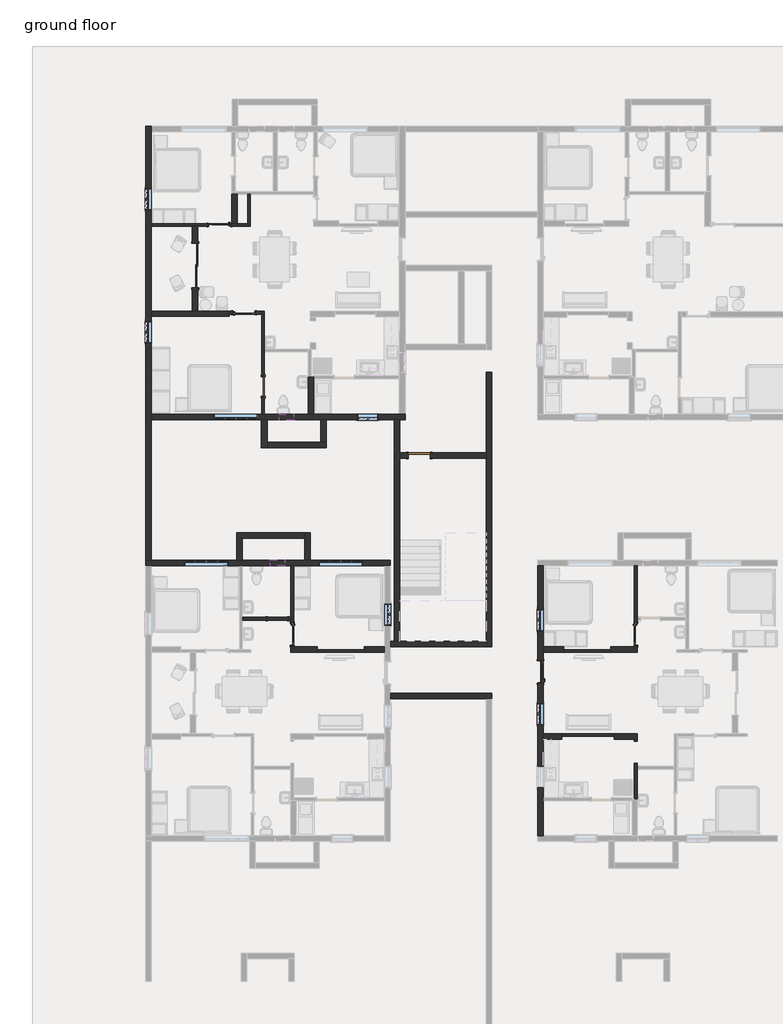
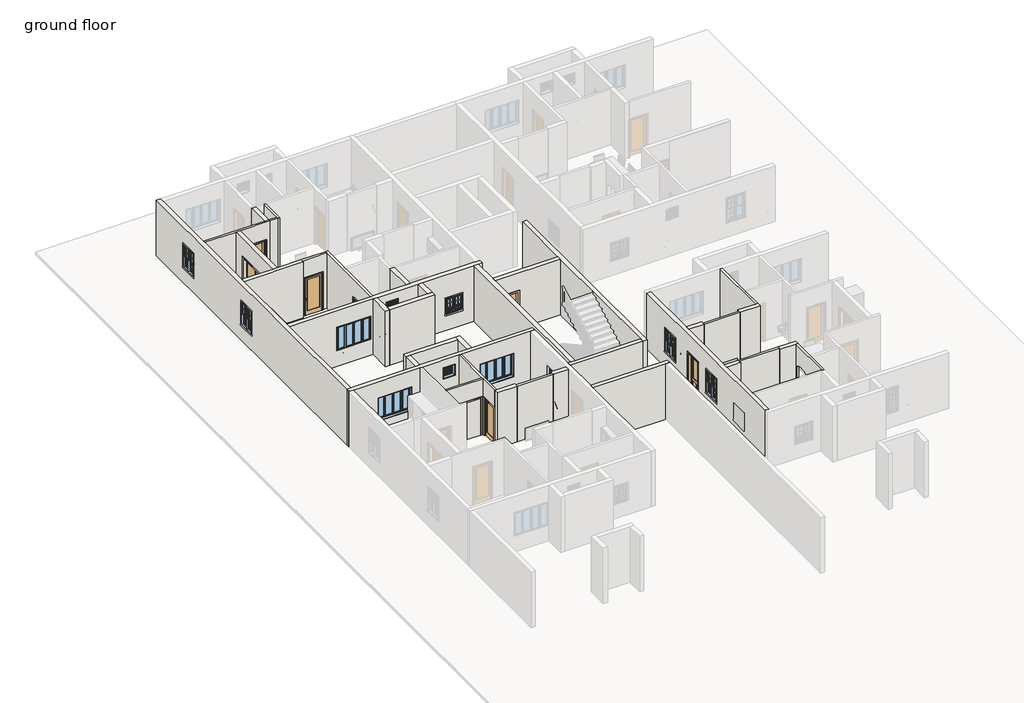
# One storey, part 7 of 16: 38 walls, 11 windows, 9 doors.
"""IFC4 building model written with IfcOpenShell, lengths in millimetres."""

from ifc_helpers import new_model, si_unit, point, frame, origin, place, context, project, spatial, polyline, ellipse_curve, trimmed, outline, extrude, faceted_brep, transform, mapped, element, save
from ifc_brep_helpers import plane_surface, extruded_surface, advanced_brep
from components import door_f079f64e, door_d4d75d1e, door_a3feeac7, door_3c6ab76a, door_38851409, door_a90ba1ad, window_ced37e8f, window_5487fb6d, window_f2d8fef0, window_45970670

model = new_model("IFC4")

# Units and contexts
model_context = context("Model", 3, world=origin())
ifc_project = project(units=[si_unit("LENGTHUNIT", "METRE", prefix="MILLI")], contexts=[model_context])

# Site, building, storey
site = spatial("IfcSite", under=ifc_project)
building = spatial("IfcBuilding", under=site)
storey = spatial("IfcBuildingStorey", under=building, Name="ground floor", Elevation=609.6)

# Doors
placement = place(None, origin())
door_shape = door_f079f64e(model_context)
element("IfcDoor", 1, ObjectType="36\" x 84\"", at=placement, inside=storey, context=model_context, shape_type="MappedRepresentation", body=[
    mapped(door_shape, transform((59474.0062819, 28018.8650652, 609.6), x_axis=(0.0, -1.0, 0.0), y_axis=(1.0, 0.0, 0.0), z_axis=(0.0, 0.0, 1.0))),
])
door_2_shape = door_d4d75d1e(model_context)
element("IfcDoor", 2, ObjectType="Door-Double-Sliding : 72\" x 84\"", at=placement, inside=storey, context=model_context, shape_type="MappedRepresentation", body=[
    mapped(door_2_shape, transform((45068.5142308, 44814.5310851, 609.6), x_axis=(0.0, -1.0, 0.0), y_axis=(1.0, 0.0, 0.0), z_axis=(0.0, 0.0, 1.0))),
])
door_3_shape = door_a3feeac7(model_context)
element("IfcDoor", 3, ObjectType="Door-Interior-Single-1_Panel-Wood : 36\" x 84\"", at=placement, inside=storey, context=model_context, shape_type="MappedRepresentation", body=[
    mapped(door_3_shape, transform((46206.3837344, 46494.1060851, 609.6), x_axis=(-1.0, 0.0, 0.0), y_axis=(0.0, -1.0, 0.0), z_axis=(0.0, 0.0, 1.0))),
])
element("IfcDoor", 4, ObjectType="Door-Interior-Single-1_Panel-Wood : 36\" x 84\"", at=placement, inside=storey, context=model_context, shape_type="MappedRepresentation", body=[
    mapped(door_3_shape, transform((47204.5368314, 42863.06804, 609.6), x_axis=(1.0, 0.0, 0.0), y_axis=(0.0, 1.0, 0.0), z_axis=(0.0, 0.0, 1.0))),
])
element("IfcDoor", 5, ObjectType="Door-Interior-Single-1_Panel-Wood : 36\" x 84\"", at=placement, inside=storey, context=model_context, shape_type="MappedRepresentation", body=[
    mapped(door_3_shape, transform((63411.0062819, 29571.4400652, 609.6), x_axis=(0.0, -1.0, 0.0), y_axis=(1.0, 0.0, 0.0), z_axis=(0.0, 0.0, 1.0))),
])
door_4_shape = door_3c6ab76a(model_context)
element("IfcDoor", 6, ObjectType="Door-Interior-Single-1_Panel-Wood : 36\" x 84\"", at=placement, inside=storey, context=model_context, shape_type="MappedRepresentation", body=[
    mapped(door_4_shape, transform((49209.051243, 29571.4400652, 609.6), x_axis=(0.0, -1.0, 0.0), y_axis=(1.0, 0.0, 0.0), z_axis=(0.0, 0.0, 1.0))),
])
door_5_shape = door_38851409(model_context)
element("IfcDoor", 7, ObjectType="Single-Flush : 32\" x 84\"", at=placement, inside=storey, context=model_context, shape_type="MappedRepresentation", body=[
    mapped(door_5_shape, transform((47998.2868314, 39817.8809867, 609.6), x_axis=(0.0, 1.0, 0.0), y_axis=(-1.0, 0.0, 0.0), z_axis=(0.0, 0.0, 1.0))),
])
element("IfcDoor", 8, ObjectType="Single-Flush : 32\" x 84\"", at=placement, inside=storey, context=model_context, shape_type="MappedRepresentation", body=[
    mapped(door_5_shape, transform((48596.276243, 30209.6150652, 609.6), x_axis=(-1.0, 0.0, 0.0), y_axis=(0.0, -1.0, 0.0), z_axis=(0.0, 0.0, 1.0))),
])
door_6_shape = door_a90ba1ad(model_context)
element("IfcDoor", 9, ObjectType="Single-Flush : 36\" x 84\"", at=placement, inside=storey, context=model_context, shape_type="MappedRepresentation", body=[
    mapped(door_6_shape, transform((54460.4072437, 36957.8375431, 609.6), x_axis=(-1.0, 0.0, 0.0), y_axis=(0.0, -1.0, 0.0), z_axis=(0.0, 0.0, 1.0))),
])

# Walls
element("IfcWall", 10, ObjectType="Generic - 4.5\"", at=placement, inside=storey, context=model_context, shape_type="Brep", body=[
    faceted_brep([(47941.1368314, 42923.39304, 609.6), (47941.1368314, 42809.09304, 609.6), (47941.1368314, 40224.2809867, 609.6), (47941.1368314, 40224.2809867, 2743.2), (47941.1368314, 39411.4809867, 2743.2), (47941.1368314, 39411.4809867, 609.6), (47941.1368314, 38662.1809867, 609.6), (47941.1368314, 38662.1809867, 3810.0), (47941.1368314, 42809.09304, 3810.0), (47941.1368314, 42923.39304, 3810.0), (48055.4368314, 40224.2809867, 2743.2), (48055.4368314, 40224.2809867, 609.6), (48055.4368314, 41243.6395295, 609.6), (48055.4368314, 41357.9395295, 609.6), (48055.4368314, 42923.39304, 609.6), (48055.4368314, 42923.39304, 3810.0), (48055.4368314, 41357.9395295, 3810.0), (48055.4368314, 41243.6395295, 3810.0), (48055.4368314, 38662.1809867, 3810.0), (48055.4368314, 38662.1809867, 609.6), (48055.4368314, 39411.4809867, 609.6), (48055.4368314, 39411.4809867, 2743.2)], [[[0, 1, 2, 3, 4, 5, 6, 7, 8, 9]], [[10, 11, 12, 13, 14, 15, 16, 17, 18, 19, 20, 21]], [[20, 19, 6, 5]], [[14, 13, 12, 11, 2, 1, 0]], [[9, 8, 7, 18, 17, 16, 15]], [[0, 9, 15, 14]], [[7, 6, 19, 18]], [[3, 2, 11, 10]], [[4, 3, 10, 21]], [[5, 4, 21, 20]]]),
])
element("IfcWall", 11, ObjectType="Generic - 4.5\"", at=placement, inside=storey, context=model_context, shape_type="SweptSolid", body=[
    extrude(outline(polyline([(3810.0, 46594.9368314), (609.6, 46594.9368314), (609.6, 46721.9368314), (2768.6, 46721.9368314), (2768.6, 47687.1368314), (609.6, 47687.1368314), (609.6, 47941.1368314), (3810.0, 47941.1368314), (3810.0, 46594.9368314)])), frame((0.0, 42809.09304, 0.0), z_axis=(0.0, 1.0, 0.0), x_axis=(0.0, 0.0, 1.0)), (0.0, 0.0, 1.0), 114.3),
])
element("IfcWall", 12, ObjectType="Generic - 4.5\"", at=placement, inside=storey, context=model_context, shape_type="Brep", body=[
    faceted_brep([(46930.2837344, 46433.7810851, 3810.0), (45309.8142308, 46433.7810851, 3810.0), (45081.2142308, 46433.7810851, 3810.0), (43370.226243, 46433.7810851, 3810.0), (43370.226243, 46433.7810851, 609.6), (45081.2142308, 46433.7810851, 609.6), (45309.8142308, 46433.7810851, 609.6), (45723.7837344, 46433.7810851, 609.6), (45723.7837344, 46433.7810851, 2768.6), (46688.9837344, 46433.7810851, 2768.6), (46688.9837344, 46433.7810851, 609.6), (46930.2837344, 46433.7810851, 609.6), (43370.226243, 46548.0810851, 3810.0), (46701.6837344, 46548.0810851, 3810.0), (46930.2837344, 46548.0810851, 3810.0), (46930.2837344, 46548.0810851, 609.6), (46701.6837344, 46548.0810851, 609.6), (46688.9837344, 46548.0810851, 609.6), (46688.9837344, 46548.0810851, 2768.6), (45723.7837344, 46548.0810851, 2768.6), (45723.7837344, 46548.0810851, 609.6), (43370.226243, 46548.0810851, 609.6)], [[[0, 1, 2, 3, 4, 5, 6, 7, 8, 9, 10, 11]], [[12, 13, 14, 15, 16, 17, 18, 19, 20, 21]], [[4, 21, 20, 7, 6, 5]], [[15, 11, 10, 17, 16]], [[3, 2, 1, 0, 14, 13, 12]], [[4, 3, 12, 21]], [[0, 11, 15, 14]], [[19, 8, 7, 20]], [[8, 19, 18, 9]], [[9, 18, 17, 10]]]),
])
element("IfcWall", 13, ObjectType="Generic - 4.5\"", at=placement, inside=storey, context=model_context, shape_type="Brep", body=[
    faceted_brep([(47362.0837344, 47759.2773256, 609.6), (47362.0837344, 46547.9632967, 609.6), (47362.0837344, 46433.6632967, 609.6), (47362.0837344, 46433.6632967, 3810.0), (47362.0837344, 46547.9632967, 3810.0), (47362.0837344, 47759.2773256, 3810.0), (47476.3837344, 47759.2773256, 609.6), (47476.3837344, 47759.2773256, 3810.0), (47476.3837344, 46433.6632967, 3810.0), (47476.3837344, 46433.6632967, 609.6)], [[[0, 1, 2, 3, 4, 5]], [[6, 7, 8, 9]], [[2, 1, 0, 6, 9]], [[5, 4, 3, 8, 7]], [[0, 5, 7, 6]], [[3, 2, 9, 8]]]),
])
element("IfcWall", 14, ObjectType="Generic - 4.5\"", at=placement, inside=storey, context=model_context, shape_type="SweptSolid", body=[
    extrude(outline(polyline([(46930.2837344, 46547.9632967), (47362.0837344, 46547.9632967), (47362.0837344, 46433.6632967), (46930.2837344, 46433.6632967), (46930.2837344, 46547.9632967)])), frame((0.0, 0.0, 609.6), z_axis=(0.0, 0.0, 1.0), x_axis=(1.0, 0.0, 0.0)), (0.0, 0.0, 1.0), 3200.4),
])
element("IfcWall", 15, ObjectType="Generic - 4.5\"", at=placement, inside=storey, context=model_context, shape_type="SweptSolid", body=[
    extrude(outline(polyline([(62518.8312819, 25351.8650652), (60347.1312819, 25351.8650652), (60347.1312819, 25466.1650652), (62518.8312819, 25466.1650652), (62518.8312819, 25351.8650652)])), frame((0.0, 0.0, 609.6), z_axis=(0.0, 0.0, 1.0), x_axis=(1.0, 0.0, 0.0)), (0.0, 0.0, 1.0), 3200.4),
])
element("IfcWall", 16, ObjectType="Generic - 4.5\"", at=placement, inside=storey, context=model_context, shape_type="AdvancedBrep", body=[
    advanced_brep(
    [(63357.0312819, 24243.7900652, 2540.0), (63357.0312819, 24243.7900652, 609.6), (63357.0312819, 22811.8650652, 609.6), (63357.0312819, 22754.7150652, 609.6), (63357.0312819, 22754.7150652, 3810.0), (63357.0312819, 22811.8650652, 3810.0), (63357.0312819, 25237.5650652, 3810.0), (63357.0312819, 25237.5650652, 609.6), (63357.0312819, 25158.1900652, 609.6), (63357.0312819, 25158.1900652, 2540.0), (63471.3312819, 22754.7150652, 609.6), (63471.3312819, 23992.9650652, 609.6), (63471.3312819, 24107.2650652, 609.6), (63471.3312819, 24243.7900652, 609.6), (63471.3312819, 24243.7900652, 2540.0), (63471.3312819, 25158.1900652, 2540.0), (63471.3312819, 25158.1900652, 609.6), (63471.3312819, 25237.5650652, 609.6), (63471.3312819, 25237.5650652, 3810.0), (63471.3312819, 24107.2650652, 3810.0), (63471.3312819, 23992.9650652, 3810.0), (63471.3312819, 22754.7150652, 3810.0)],
    [
        (0, 1),
        (1, 2),
        (2, 3),
        (3, 4),
        (4, 5),
        (5, 6),
        (6, 7),
        (7, 8),
        (8, 9),
        (9, 0, ellipse_curve(frame((63357.0312819, 24700.9900652, 2540.0), z_axis=(1.0, 0.0, 0.0), x_axis=(0.0, -1.0, 0.0)), 457.2, 203.2)),
        (10, 11),
        (11, 12),
        (12, 13),
        (13, 14),
        (14, 15, ellipse_curve(frame((63471.3312819, 24700.9900652, 2540.0), z_axis=(-1.0, 0.0, 0.0), x_axis=(0.0, -1.0, 0.0)), 457.2, 203.2)),
        (15, 16),
        (16, 17),
        (17, 18),
        (18, 19),
        (19, 20),
        (20, 21),
        (21, 10),
        (7, 17),
        (16, 8),
        (1, 13),
        (10, 3),
        (21, 4),
        (18, 6),
        (14, 0),
        (9, 15),
    ],
    [
        plane_surface(frame((63357.0312819, 25237.5650652, 609.6), z_axis=(-1.0, 0.0, 0.0), x_axis=(0.0, -1.0, 0.0))),
        plane_surface(frame((63471.3312819, 25237.5650652, 609.6), z_axis=(1.0, 0.0, 0.0), x_axis=(0.0, 1.0, 0.0))),
        plane_surface(frame((63357.0312819, 25351.8650652, 609.6), z_axis=(0.0, 0.0, -1.0), x_axis=(1.0, 0.0, 0.0))),
        plane_surface(frame((63357.0312819, 22754.7150652, 609.6), z_axis=(0.0, -1.0, 0.0), x_axis=(1.0, 0.0, 0.0))),
        plane_surface(frame((63357.0312819, 22754.7150652, 3810.0), z_axis=(0.0, 0.0, 1.0), x_axis=(1.0, 0.0, 0.0))),
        plane_surface(frame((62518.8312819, 25237.5650652, 609.6), z_axis=(0.0, 1.0, 0.0), x_axis=(1.0, 0.0, 0.0))),
        extruded_surface(trimmed(ellipse_curve(frame((63242.7312819, 24700.9900652, 2540.0), z_axis=(-1.0, 0.0, 0.0), x_axis=(0.0, -1.0, 0.0)), 457.2, 203.2), [point((63242.7312819, 24243.7900652, 2540.0))], [point((63242.7312819, 25158.1900652, 2540.0))], True, "CARTESIAN"), (114.30000000000291, 0.0, 0.0), 114.30000000000291),
        plane_surface(frame((63471.3312819, 25158.1900652, 2540.0), z_axis=(0.0, -1.0, 0.0), x_axis=(-1.0, 0.0, 0.0))),
        plane_surface(frame((63471.3312819, 24243.7900652, 609.6), z_axis=(0.0, 1.0, 0.0), x_axis=(-1.0, 0.0, 0.0))),
    ],
    [
        (0, [[1, 2, 3, 4, 5, 6, 7, 8, 9, 10]]),
        (1, [[11, 12, 13, 14, 15, 16, 17, 18, 19, 20, 21, 22]]),
        (2, [[-8, 23, -17, 24]]),
        (2, [[-3, -2, 25, -13, -12, -11, 26]]),
        (3, [[-4, -26, -22, 27]]),
        (4, [[-6, -5, -27, -21, -20, -19, 28]]),
        (5, [[-7, -28, -18, -23]]),
        (6, [[-15, 29, -10, 30]]),
        (7, [[-16, -30, -9, -24]]),
        (8, [[-14, -25, -1, -29]]),
    ],
),
])
element("IfcWall", 17, ObjectType="Generic - 4.5\"", at=placement, inside=storey, context=model_context, shape_type="SweptSolid", body=[
    extrude(outline(polyline([(62384.5498476, 28818.9650652), (60423.3312819, 28818.9650652), (60423.3312819, 28933.2650652), (62384.5498476, 28933.2650652), (62384.5498476, 28818.9650652)])), frame((0.0, 0.0, 609.6), z_axis=(0.0, 0.0, 1.0), x_axis=(1.0, 0.0, 0.0)), (0.0, 0.0, 1.0), 3200.4),
])
element("IfcWall", 18, ObjectType="Generic - 4.5\"", at=placement, inside=storey, context=model_context, shape_type="Brep", body=[
    faceted_brep([(63357.0312819, 29047.5650652, 3810.0), (63357.0312819, 32400.3650652, 3810.0), (63357.0312819, 32400.3650652, 609.6), (63357.0312819, 30054.0400652, 609.6), (63357.0312819, 30054.0400652, 2768.6), (63357.0312819, 29088.8400652, 2768.6), (63357.0312819, 29088.8400652, 609.6), (63357.0312819, 29047.5650652, 609.6), (63471.3312819, 32400.3650652, 3810.0), (63471.3312819, 30266.7650652, 3810.0), (63471.3312819, 30152.4650652, 3810.0), (63471.3312819, 29047.5650652, 3810.0), (63471.3312819, 29047.5650652, 609.6), (63471.3312819, 29088.8400652, 609.6), (63471.3312819, 29088.8400652, 2768.6), (63471.3312819, 30054.0400652, 2768.6), (63471.3312819, 30054.0400652, 609.6), (63471.3312819, 30152.4650652, 609.6), (63471.3312819, 30266.7650652, 609.6), (63471.3312819, 32400.3650652, 609.6)], [[[0, 1, 2, 3, 4, 5, 6, 7]], [[8, 9, 10, 11, 12, 13, 14, 15, 16, 17, 18, 19]], [[2, 19, 18, 17, 16, 3]], [[12, 7, 6, 13]], [[1, 0, 11, 10, 9, 8]], [[0, 7, 12, 11]], [[2, 1, 8, 19]], [[5, 14, 13, 6]], [[14, 5, 4, 15]], [[15, 4, 3, 16]]]),
])
element("IfcWall", 19, ObjectType="Generic - 4.5\"", at=placement, inside=storey, context=model_context, shape_type="Brep", body=[
    faceted_brep([(49148.726243, 29047.5650652, 3810.0), (49148.726243, 30152.4650652, 3810.0), (49148.726243, 30266.7650652, 3810.0), (49148.726243, 32412.9272014, 3810.0), (49148.726243, 32412.9272014, 609.6), (49148.726243, 30266.7650652, 609.6), (49148.726243, 30152.4650652, 609.6), (49148.726243, 30054.0400652, 609.6), (49148.726243, 30054.0400652, 2768.6), (49148.726243, 29088.8400652, 2768.6), (49148.726243, 29088.8400652, 609.6), (49148.726243, 29047.5650652, 609.6), (49263.026243, 32412.9272014, 3810.0), (49263.026243, 29047.5650652, 3810.0), (49263.026243, 29047.5650652, 609.6), (49263.026243, 29088.8400652, 609.6), (49263.026243, 29088.8400652, 2768.6), (49263.026243, 30054.0400652, 2768.6), (49263.026243, 30054.0400652, 609.6), (49263.026243, 32412.9272014, 609.6)], [[[0, 1, 2, 3, 4, 5, 6, 7, 8, 9, 10, 11]], [[12, 13, 14, 15, 16, 17, 18, 19]], [[4, 19, 18, 7, 6, 5]], [[14, 11, 10, 15]], [[3, 2, 1, 0, 13, 12]], [[0, 11, 14, 13]], [[4, 3, 12, 19]], [[9, 16, 15, 10]], [[16, 9, 8, 17]], [[17, 8, 7, 18]]]),
])
element("IfcWall", 20, ObjectType="Generic - 4.5\"", at=placement, inside=storey, context=model_context, shape_type="SweptSolid", body=[
    extrude(outline(polyline([(49148.726243, 30152.4650652), (47142.126243, 30152.4650652), (47142.126243, 30266.7650652), (49148.726243, 30266.7650652), (49148.726243, 30152.4650652)])), frame((0.0, 0.0, 609.6), z_axis=(0.0, 0.0, 1.0), x_axis=(1.0, 0.0, 0.0)), (0.0, 0.0, 1.0), 3200.4),
])
element("IfcWall", 21, ObjectType="Generic - 4.5\"", at=placement, inside=storey, context=model_context, shape_type="SweptSolid", body=[
    extrude(outline(polyline([(52192.1804737, 28818.9650652), (50235.5076773, 28818.9650652), (50235.5076773, 28933.2650652), (52192.1804737, 28933.2650652), (52192.1804737, 28818.9650652)])), frame((0.0, 0.0, 609.6), z_axis=(0.0, 0.0, 1.0), x_axis=(1.0, 0.0, 0.0)), (0.0, 0.0, 1.0), 3200.4),
])
element("IfcWall", 22, ObjectType="Generic - 4.5\"", at=placement, inside=storey, context=model_context, shape_type="SweptSolid", body=[
    extrude(outline(polyline([(609.6, 47142.126243), (609.6, 48189.876243), (2743.2, 48189.876243), (2743.2, 49002.676243), (609.6, 49002.676243), (609.6, 49148.726243), (3810.0, 49148.726243), (3810.0, 47142.126243), (609.6, 47142.126243)])), frame((0.0, 30152.4650652, 0.0), z_axis=(0.0, 1.0, 0.0), x_axis=(0.0, 0.0, 1.0)), (0.0, 0.0, 1.0), 114.3),
])
element("IfcWall", 23, ObjectType="Generic - 8\"", at=placement, inside=storey, context=model_context, shape_type="Brep", body=[
    faceted_brep([(43370.226243, 42720.1903135, 609.6), (46594.9368314, 42720.1903135, 609.6), (46594.9368314, 42720.1903135, 3810.0), (43370.226243, 42720.1903135, 3810.0), (43370.226243, 42923.3903135, 609.6), (43370.226243, 42923.3903135, 3810.0), (45081.2142308, 42923.3903135, 3810.0), (45309.8142308, 42923.3903135, 3810.0), (46594.9368314, 42923.3903135, 3810.0), (46594.9368314, 42923.3903135, 609.6), (45309.8142308, 42923.3903135, 609.6), (45081.2142308, 42923.3903135, 609.6), (46594.9368314, 42809.09304, 609.6), (46594.9368314, 42809.09304, 3810.0)], [[[0, 1, 2, 3]], [[4, 5, 6, 7, 8, 9, 10, 11]], [[1, 0, 4, 11, 10, 9, 12]], [[2, 1, 12, 9, 8, 13]], [[3, 2, 13, 8, 7, 6, 5]], [[0, 3, 5, 4]]]),
])
element("IfcWall", 24, ObjectType="Generic - 9\"", at=placement, inside=storey, context=model_context, shape_type="Brep", body=[
    faceted_brep([(43141.626243, 50583.0390836, 609.6), (43141.626243, 32641.5272014, 609.6), (43141.626243, 32641.5272014, 3810.0), (43141.626243, 50583.0390836, 3810.0), (43141.626243, 41602.5903135, 2844.8), (43141.626243, 41602.5903135, 1524.0), (43141.626243, 42516.9903135, 1524.0), (43141.626243, 42516.9903135, 2844.8), (43141.626243, 47100.5310851, 2844.8), (43141.626243, 47100.5310851, 1524.0), (43141.626243, 48014.9310851, 1524.0), (43141.626243, 48014.9310851, 2844.8), (43370.226243, 50583.0390836, 609.6), (43370.226243, 50583.0390836, 3810.0), (43370.226243, 50354.4390836, 3810.0), (43370.226243, 46548.0810851, 3810.0), (43370.226243, 46433.7810851, 3810.0), (43370.226243, 42923.3903135, 3810.0), (43370.226243, 42720.1903135, 3810.0), (43370.226243, 38662.1809867, 3810.0), (43370.226243, 38433.5809867, 3810.0), (43370.226243, 32641.5272014, 3810.0), (43370.226243, 32641.5272014, 609.6), (43370.226243, 38433.5809867, 609.6), (43370.226243, 38662.1809867, 609.6), (43370.226243, 42720.1903135, 609.6), (43370.226243, 42923.3903135, 609.6), (43370.226243, 46433.7810851, 609.6), (43370.226243, 46548.0810851, 609.6), (43370.226243, 50354.4390836, 609.6), (43370.226243, 41602.5903135, 2844.8), (43370.226243, 42516.9903135, 2844.8), (43370.226243, 42516.9903135, 1524.0), (43370.226243, 41602.5903135, 1524.0), (43370.226243, 47100.5310851, 2844.8), (43370.226243, 48014.9310851, 2844.8), (43370.226243, 48014.9310851, 1524.0), (43370.226243, 47100.5310851, 1524.0)], [[[0, 1, 2, 3], [4, 5, 6, 7], [8, 9, 10, 11]], [[12, 13, 14, 15, 16, 17, 18, 19, 20, 21, 22, 23, 24, 25, 26, 27, 28, 29], [30, 31, 32, 33], [34, 35, 36, 37]], [[1, 0, 12, 29, 28, 27, 26, 25, 24, 23, 22]], [[3, 2, 21, 20, 19, 18, 17, 16, 15, 14, 13]], [[0, 3, 13, 12]], [[5, 4, 30, 33]], [[6, 5, 33, 32]], [[7, 6, 32, 31]], [[4, 7, 31, 30]], [[9, 8, 34, 37]], [[10, 9, 37, 36]], [[11, 10, 36, 35]], [[8, 11, 35, 34]], [[2, 1, 22, 21]]]),
])
element("IfcWall", 25, ObjectType="Generic - 9\"", at=placement, inside=storey, context=model_context, shape_type="Brep", body=[
    faceted_brep([(43370.226243, 38433.5809867, 609.6), (47935.8141396, 38433.5809867, 609.6), (48164.4141396, 38433.5809867, 609.6), (50387.9122064, 38433.5809867, 609.6), (50616.5122064, 38433.5809867, 609.6), (53431.7072437, 38433.5809867, 609.6), (53660.3072437, 38433.5809867, 609.6), (53870.1312819, 38433.5809867, 609.6), (53870.1312819, 38433.5809867, 3810.0), (53660.3072437, 38433.5809867, 3810.0), (53431.7072437, 38433.5809867, 3810.0), (50616.5122064, 38433.5809867, 3810.0), (50387.9122064, 38433.5809867, 3810.0), (48164.4141396, 38433.5809867, 3810.0), (47935.8141396, 38433.5809867, 3810.0), (43370.226243, 38433.5809867, 3810.0), (49269.3141396, 38433.5809867, 3352.8), (49269.3141396, 38433.5809867, 2743.2), (48659.7141396, 38433.5809867, 2743.2), (48659.7141396, 38433.5809867, 3352.8), (45966.2868314, 38433.5809867, 1524.0), (45966.2868314, 38433.5809867, 2870.2), (47795.0868314, 38433.5809867, 2870.2), (47795.0868314, 38433.5809867, 1524.0), (51901.6312819, 38433.5809867, 1524.0), (51901.6312819, 38433.5809867, 2438.4), (52765.2312819, 38433.5809867, 2438.4), (52765.2312819, 38433.5809867, 1524.0), (53870.1312819, 38662.1809867, 609.6), (53641.5312819, 38662.1809867, 609.6), (50099.858718, 38662.1809867, 609.6), (49871.258718, 38662.1809867, 609.6), (48055.4368314, 38662.1809867, 609.6), (47941.1368314, 38662.1809867, 609.6), (43370.226243, 38662.1809867, 609.6), (43370.226243, 38662.1809867, 3810.0), (47941.1368314, 38662.1809867, 3810.0), (48055.4368314, 38662.1809867, 3810.0), (49871.258718, 38662.1809867, 3810.0), (50099.858718, 38662.1809867, 3810.0), (53641.5312819, 38662.1809867, 3810.0), (53870.1312819, 38662.1809867, 3810.0), (49269.3141396, 38662.1809867, 2743.2), (49269.3141396, 38662.1809867, 3352.8), (48659.7141396, 38662.1809867, 3352.8), (48659.7141396, 38662.1809867, 2743.2), (45966.2868314, 38662.1809867, 2870.2), (45966.2868314, 38662.1809867, 1524.0), (47795.0868314, 38662.1809867, 1524.0), (47795.0868314, 38662.1809867, 2870.2), (51901.6312819, 38662.1809867, 2438.4), (51901.6312819, 38662.1809867, 1524.0), (52765.2312819, 38662.1809867, 1524.0), (52765.2312819, 38662.1809867, 2438.4)], [[[0, 1, 2, 3, 4, 5, 6, 7, 8, 9, 10, 11, 12, 13, 14, 15], [16, 17, 18, 19], [20, 21, 22, 23], [24, 25, 26, 27]], [[28, 29, 30, 31, 32, 33, 34, 35, 36, 37, 38, 39, 40, 41], [42, 43, 44, 45], [46, 47, 48, 49], [50, 51, 52, 53]], [[7, 6, 5, 4, 3, 2, 1, 0, 34, 33, 32, 31, 30, 29, 28]], [[15, 14, 13, 12, 11, 10, 9, 8, 41, 40, 39, 38, 37, 36, 35]], [[0, 15, 35, 34]], [[8, 7, 28, 41]], [[17, 16, 43, 42]], [[18, 17, 42, 45]], [[19, 18, 45, 44]], [[16, 19, 44, 43]], [[47, 46, 21, 20]], [[48, 47, 20, 23]], [[49, 48, 23, 22]], [[46, 49, 22, 21]], [[50, 25, 24, 51]], [[51, 24, 27, 52]], [[52, 27, 26, 53]], [[25, 50, 53, 26]]]),
])
element("IfcWall", 26, ObjectType="Generic - 9\"", at=placement, inside=storey, context=model_context, shape_type="SweptSolid", body=[
    extrude(outline(polyline([(43900.1310851, 2743.2), (43900.1310851, 609.6), (42923.3903135, 609.6), (42923.3903135, 3810.0), (46433.7810851, 3810.0), (46433.7810851, 609.6), (45728.9310851, 609.6), (45728.9310851, 2743.2), (43900.1310851, 2743.2)])), frame((45081.2142308, 0.0, 0.0), z_axis=(1.0, 0.0, 0.0), x_axis=(0.0, 1.0, 0.0)), (0.0, 0.0, 1.0), 228.6),
])
element("IfcWall", 27, ObjectType="Generic - 9\"", at=placement, inside=storey, context=model_context, shape_type="Brep", body=[
    faceted_brep([(50099.858718, 38662.1809867, 609.6), (50099.858718, 40142.3043028, 609.6), (50099.858718, 40199.4543028, 609.6), (50099.858718, 40199.4543028, 3810.0), (50099.858718, 40142.3043028, 3810.0), (50099.858718, 38662.1809867, 3810.0), (49871.258718, 38662.1809867, 609.6), (49871.258718, 38662.1809867, 3810.0), (49871.258718, 40199.4543028, 3810.0), (49871.258718, 40199.4543028, 609.6), (49985.558718, 40199.4543028, 609.6), (49985.558718, 40199.4543028, 3810.0)], [[[0, 1, 2, 3, 4, 5]], [[6, 7, 8, 9]], [[2, 1, 0, 6, 9, 10]], [[3, 2, 10, 9, 8, 11]], [[5, 4, 3, 11, 8, 7]], [[0, 5, 7, 6]]]),
])
element("IfcWall", 28, ObjectType="Generic - 9\"", at=placement, inside=storey, context=model_context, shape_type="SweptSolid", body=[
    extrude(outline(polyline([(46930.2837344, 47759.2773256), (46930.2837344, 46548.0810851), (46701.6837344, 46548.0810851), (46701.6837344, 47759.2773256), (46930.2837344, 47759.2773256)])), frame((0.0, 0.0, 609.6), z_axis=(0.0, 0.0, 1.0), x_axis=(1.0, 0.0, 0.0)), (0.0, 0.0, 1.0), 3200.4),
])
element("IfcWall", 29, ObjectType="Generic - 9\"", at=placement, inside=storey, context=model_context, shape_type="Brep", body=[
    faceted_brep([(47935.8141396, 38433.5809867, 609.6), (47935.8141396, 37283.0593578, 609.6), (47935.8141396, 37283.0593578, 3810.0), (47935.8141396, 38433.5809867, 3810.0), (48164.4141396, 38433.5809867, 609.6), (48164.4141396, 38433.5809867, 3810.0), (48164.4141396, 37511.6593578, 3810.0), (48164.4141396, 37283.0593578, 3810.0), (48164.4141396, 37283.0593578, 609.6), (48164.4141396, 37511.6593578, 609.6)], [[[0, 1, 2, 3]], [[4, 5, 6, 7, 8, 9]], [[1, 0, 4, 9, 8]], [[3, 2, 7, 6, 5]], [[0, 3, 5, 4]], [[2, 1, 8, 7]]]),
])
element("IfcWall", 30, ObjectType="Generic - 9\"", at=placement, inside=storey, context=model_context, shape_type="Brep", body=[
    faceted_brep([(48164.4141396, 37283.0593578, 609.6), (50616.5122064, 37283.0593578, 609.6), (50616.5122064, 37283.0593578, 3810.0), (48164.4141396, 37283.0593578, 3810.0), (48164.4141396, 37511.6593578, 609.6), (48164.4141396, 37511.6593578, 3810.0), (50387.9122064, 37511.6593578, 3810.0), (50616.5122064, 37511.6593578, 3810.0), (50616.5122064, 37511.6593578, 609.6), (50387.9122064, 37511.6593578, 609.6)], [[[0, 1, 2, 3]], [[4, 5, 6, 7, 8, 9]], [[1, 0, 4, 9, 8]], [[3, 2, 7, 6, 5]], [[0, 3, 5, 4]], [[2, 1, 8, 7]]]),
])
element("IfcWall", 31, ObjectType="Generic - 9\"", at=placement, inside=storey, context=model_context, shape_type="SweptSolid", body=[
    extrude(outline(polyline([(50616.5122064, 38433.5809867), (50616.5122064, 37511.6593578), (50387.9122064, 37511.6593578), (50387.9122064, 38433.5809867), (50616.5122064, 38433.5809867)])), frame((0.0, 0.0, 609.6), z_axis=(0.0, 0.0, 1.0), x_axis=(1.0, 0.0, 0.0)), (0.0, 0.0, 1.0), 3200.4),
])
element("IfcWall", 32, ObjectType="Generic - 9\"", at=placement, inside=storey, context=model_context, shape_type="Brep", body=[
    faceted_brep([(59585.1312819, 32400.3650652, 3810.0), (59585.1312819, 29047.5650652, 3810.0), (59585.1312819, 28818.9650652, 3810.0), (59585.1312819, 25466.1650652, 3810.0), (59585.1312819, 25237.5650652, 3810.0), (59585.1312819, 22811.8650652, 3810.0), (59585.1312819, 22697.5650652, 3810.0), (59585.1312819, 21249.7650652, 3810.0), (59585.1312819, 21249.7650652, 609.6), (59585.1312819, 22697.5650652, 609.6), (59585.1312819, 22811.8650652, 609.6), (59585.1312819, 25237.5650652, 609.6), (59585.1312819, 25466.1650652, 609.6), (59585.1312819, 27536.2650652, 609.6), (59585.1312819, 27536.2650652, 2768.6), (59585.1312819, 28501.4650652, 2768.6), (59585.1312819, 28501.4650652, 609.6), (59585.1312819, 28818.9650652, 609.6), (59585.1312819, 29047.5650652, 609.6), (59585.1312819, 32400.3650652, 609.6), (59585.1312819, 25809.0650652, 2844.8), (59585.1312819, 26723.4650652, 2844.8), (59585.1312819, 26723.4650652, 1524.0), (59585.1312819, 25809.0650652, 1524.0), (59585.1312819, 29695.2650652, 2844.8), (59585.1312819, 30609.6650652, 2844.8), (59585.1312819, 30609.6650652, 1524.0), (59585.1312819, 29695.2650652, 1524.0), (59585.1312819, 24100.9150652, 2438.4), (59585.1312819, 24100.9150652, 1524.0), (59585.1312819, 23237.3150652, 1524.0), (59585.1312819, 23237.3150652, 2438.4), (59356.5312819, 21249.7650652, 3810.0), (59356.5312819, 32400.3650652, 3810.0), (59356.5312819, 32400.3650652, 609.6), (59356.5312819, 28501.4650652, 609.6), (59356.5312819, 28501.4650652, 2768.6), (59356.5312819, 27536.2650652, 2768.6), (59356.5312819, 27536.2650652, 609.6), (59356.5312819, 21249.7650652, 609.6), (59356.5312819, 25809.0650652, 2844.8), (59356.5312819, 25809.0650652, 1524.0), (59356.5312819, 26723.4650652, 1524.0), (59356.5312819, 26723.4650652, 2844.8), (59356.5312819, 29695.2650652, 2844.8), (59356.5312819, 29695.2650652, 1524.0), (59356.5312819, 30609.6650652, 1524.0), (59356.5312819, 30609.6650652, 2844.8), (59356.5312819, 24100.9150652, 2438.4), (59356.5312819, 23237.3150652, 2438.4), (59356.5312819, 23237.3150652, 1524.0), (59356.5312819, 24100.9150652, 1524.0)], [[[0, 1, 2, 3, 4, 5, 6, 7, 8, 9, 10, 11, 12, 13, 14, 15, 16, 17, 18, 19], [20, 21, 22, 23], [24, 25, 26, 27], [28, 29, 30, 31]], [[32, 33, 34, 35, 36, 37, 38, 39], [40, 41, 42, 43], [44, 45, 46, 47], [48, 49, 50, 51]], [[8, 39, 38, 13, 12, 11, 10, 9]], [[34, 19, 18, 17, 16, 35]], [[7, 6, 5, 4, 3, 2, 1, 0, 33, 32]], [[0, 19, 34, 33]], [[8, 7, 32, 39]], [[37, 14, 13, 38]], [[14, 37, 36, 15]], [[15, 36, 35, 16]], [[41, 40, 20, 23]], [[42, 41, 23, 22]], [[43, 42, 22, 21]], [[40, 43, 21, 20]], [[45, 44, 24, 27]], [[46, 45, 27, 26]], [[47, 46, 26, 25]], [[44, 47, 25, 24]], [[29, 28, 48, 51]], [[30, 29, 51, 50]], [[31, 30, 50, 49]], [[28, 31, 49, 48]]]),
])
element("IfcWall", 33, ObjectType="Generic - 9\"", at=placement, inside=storey, context=model_context, shape_type="Brep", body=[
    faceted_brep([(59585.1312819, 28818.9650652, 609.6), (60423.3312819, 28818.9650652, 609.6), (60423.3312819, 28818.9650652, 3810.0), (59585.1312819, 28818.9650652, 3810.0), (59585.1312819, 29047.5650652, 609.6), (59585.1312819, 29047.5650652, 3810.0), (60423.3312819, 29047.5650652, 3810.0), (60423.3312819, 29047.5650652, 609.6), (60423.3312819, 28933.2650652, 609.6), (60423.3312819, 28933.2650652, 3810.0)], [[[0, 1, 2, 3]], [[4, 5, 6, 7]], [[1, 0, 4, 7, 8]], [[2, 1, 8, 7, 6, 9]], [[3, 2, 9, 6, 5]], [[0, 3, 5, 4]]]),
])
element("IfcWall", 34, ObjectType="Generic - 9\"", at=placement, inside=storey, context=model_context, shape_type="Brep", body=[
    faceted_brep([(62384.5498476, 28818.9650652, 609.6), (63471.3312819, 28818.9650652, 609.6), (63471.3312819, 28818.9650652, 3810.0), (62384.5498476, 28818.9650652, 3810.0), (62384.5498476, 29047.5650652, 609.6), (62384.5498476, 29047.5650652, 3810.0), (63357.0312819, 29047.5650652, 3810.0), (63471.3312819, 29047.5650652, 3810.0), (63471.3312819, 29047.5650652, 609.6), (63357.0312819, 29047.5650652, 609.6), (62384.5498476, 28933.2650652, 609.6), (62384.5498476, 28933.2650652, 3810.0)], [[[0, 1, 2, 3]], [[4, 5, 6, 7, 8, 9]], [[1, 0, 10, 4, 9, 8]], [[3, 2, 7, 6, 5, 11]], [[0, 3, 11, 5, 4, 10]], [[2, 1, 8, 7]]]),
])
element("IfcWall", 35, ObjectType="Generic - 9\"", at=placement, inside=storey, context=model_context, shape_type="Brep", body=[
    faceted_brep([(59585.1312819, 25237.5650652, 609.6), (60347.1312819, 25237.5650652, 609.6), (60347.1312819, 25237.5650652, 3810.0), (59585.1312819, 25237.5650652, 3810.0), (59585.1312819, 25466.1650652, 609.6), (59585.1312819, 25466.1650652, 3810.0), (60347.1312819, 25466.1650652, 3810.0), (60347.1312819, 25466.1650652, 609.6), (60347.1312819, 25351.8650652, 609.6), (60347.1312819, 25351.8650652, 3810.0)], [[[0, 1, 2, 3]], [[4, 5, 6, 7]], [[1, 0, 4, 7, 8]], [[2, 1, 8, 7, 6, 9]], [[3, 2, 9, 6, 5]], [[0, 3, 5, 4]]]),
])
element("IfcWall", 36, ObjectType="Generic - 9\"", at=placement, inside=storey, context=model_context, shape_type="Brep", body=[
    faceted_brep([(62518.8312819, 25237.5650652, 609.6), (63357.0312819, 25237.5650652, 609.6), (63471.3312819, 25237.5650652, 609.6), (63471.3312819, 25237.5650652, 3810.0), (63357.0312819, 25237.5650652, 3810.0), (62518.8312819, 25237.5650652, 3810.0), (62518.8312819, 25466.1650652, 609.6), (62518.8312819, 25466.1650652, 3810.0), (63471.3312819, 25466.1650652, 3810.0), (63471.3312819, 25466.1650652, 609.6), (62518.8312819, 25351.8650652, 609.6), (62518.8312819, 25351.8650652, 3810.0)], [[[0, 1, 2, 3, 4, 5]], [[6, 7, 8, 9]], [[2, 1, 0, 10, 6, 9]], [[5, 4, 3, 8, 7, 11]], [[0, 5, 11, 7, 6, 10]], [[3, 2, 9, 8]]]),
])
element("IfcWall", 37, ObjectType="Generic - 9\"", at=placement, inside=storey, context=model_context, shape_type="Brep", body=[
    faceted_brep([(43141.626243, 32412.9272014, 609.6), (43370.226243, 32412.9272014, 609.6), (47027.826243, 32412.9272014, 609.6), (47142.126243, 32412.9272014, 609.6), (49148.726243, 32412.9272014, 609.6), (49263.026243, 32412.9272014, 609.6), (53034.926243, 32412.9272014, 609.6), (53263.526243, 32412.9272014, 609.6), (53263.526243, 32412.9272014, 3810.0), (53034.926243, 32412.9272014, 3810.0), (49263.026243, 32412.9272014, 3810.0), (49148.726243, 32412.9272014, 3810.0), (47142.126243, 32412.9272014, 3810.0), (47027.826243, 32412.9272014, 3810.0), (43370.226243, 32412.9272014, 3810.0), (43141.626243, 32412.9272014, 3810.0), (46570.626243, 32412.9272014, 2870.2), (46570.626243, 32412.9272014, 1524.0), (44741.826243, 32412.9272014, 1524.0), (44741.826243, 32412.9272014, 2870.2), (52128.0383087, 32412.9272014, 2870.2), (52128.0383087, 32412.9272014, 1524.0), (50299.2383087, 32412.9272014, 1524.0), (50299.2383087, 32412.9272014, 2870.2), (48291.476243, 32412.9272014, 3352.8), (48901.076243, 32412.9272014, 3352.8), (48901.076243, 32412.9272014, 2743.2), (48291.476243, 32412.9272014, 2743.2), (43141.626243, 32641.5272014, 609.6), (43141.626243, 32641.5272014, 3810.0), (43370.226243, 32641.5272014, 3810.0), (46913.526243, 32641.5272014, 3810.0), (47142.126243, 32641.5272014, 3810.0), (49727.7383087, 32641.5272014, 3810.0), (49956.3383087, 32641.5272014, 3810.0), (53263.526243, 32641.5272014, 3810.0), (53263.526243, 32641.5272014, 609.6), (49956.3383087, 32641.5272014, 609.6), (49727.7383087, 32641.5272014, 609.6), (47142.126243, 32641.5272014, 609.6), (46913.526243, 32641.5272014, 609.6), (43370.226243, 32641.5272014, 609.6), (46570.626243, 32641.5272014, 2870.2), (44741.826243, 32641.5272014, 2870.2), (44741.826243, 32641.5272014, 1524.0), (46570.626243, 32641.5272014, 1524.0), (52128.0383087, 32641.5272014, 2870.2), (50299.2383087, 32641.5272014, 2870.2), (50299.2383087, 32641.5272014, 1524.0), (52128.0383087, 32641.5272014, 1524.0), (48291.476243, 32641.5272014, 3352.8), (48291.476243, 32641.5272014, 2743.2), (48901.076243, 32641.5272014, 2743.2), (48901.076243, 32641.5272014, 3352.8)], [[[0, 1, 2, 3, 4, 5, 6, 7, 8, 9, 10, 11, 12, 13, 14, 15], [16, 17, 18, 19], [20, 21, 22, 23], [24, 25, 26, 27]], [[28, 29, 30, 31, 32, 33, 34, 35, 36, 37, 38, 39, 40, 41], [42, 43, 44, 45], [46, 47, 48, 49], [50, 51, 52, 53]], [[7, 6, 5, 4, 3, 2, 1, 0, 28, 41, 40, 39, 38, 37, 36]], [[15, 14, 13, 12, 11, 10, 9, 8, 35, 34, 33, 32, 31, 30, 29]], [[8, 7, 36, 35]], [[0, 15, 29, 28]], [[17, 16, 42, 45]], [[18, 17, 45, 44]], [[19, 18, 44, 43]], [[16, 19, 43, 42]], [[21, 20, 46, 49]], [[22, 21, 49, 48]], [[23, 22, 48, 47]], [[20, 23, 47, 46]], [[51, 50, 24, 27]], [[52, 51, 27, 26]], [[53, 52, 26, 25]], [[50, 53, 25, 24]]]),
])
element("IfcWall", 38, ObjectType="Generic - 9\"", at=placement, inside=storey, context=model_context, shape_type="Brep", body=[
    faceted_brep([(53034.926243, 29047.5650652, 609.6), (52192.1804737, 29047.5650652, 609.6), (52192.1804737, 29047.5650652, 3810.0), (53034.926243, 29047.5650652, 3810.0), (53034.926243, 28818.9650652, 609.6), (53034.926243, 28818.9650652, 3810.0), (52192.1804737, 28818.9650652, 3810.0), (52192.1804737, 28818.9650652, 609.6), (52192.1804737, 28933.2650652, 609.6), (52192.1804737, 28933.2650652, 3810.0)], [[[0, 1, 2, 3]], [[4, 5, 6, 7]], [[1, 0, 4, 7, 8]], [[2, 1, 8, 7, 6, 9]], [[3, 2, 9, 6, 5]], [[0, 3, 5, 4]]]),
])
element("IfcWall", 39, ObjectType="Generic - 9\"", at=placement, inside=storey, context=model_context, shape_type="Brep", body=[
    faceted_brep([(50235.5076773, 29047.5650652, 609.6), (49263.026243, 29047.5650652, 609.6), (49148.726243, 29047.5650652, 609.6), (49148.726243, 29047.5650652, 3810.0), (49263.026243, 29047.5650652, 3810.0), (50235.5076773, 29047.5650652, 3810.0), (50235.5076773, 28818.9650652, 609.6), (50235.5076773, 28818.9650652, 3810.0), (49148.726243, 28818.9650652, 3810.0), (49148.726243, 28818.9650652, 609.6), (50235.5076773, 28933.2650652, 609.6), (50235.5076773, 28933.2650652, 3810.0)], [[[0, 1, 2, 3, 4, 5]], [[6, 7, 8, 9]], [[2, 1, 0, 10, 6, 9]], [[5, 4, 3, 8, 7, 11]], [[0, 5, 11, 7, 6, 10]], [[3, 2, 9, 8]]]),
])
element("IfcWall", 40, ObjectType="Generic - 9\"", at=placement, inside=storey, context=model_context, shape_type="Brep", body=[
    faceted_brep([(57222.9312819, 40412.2375431, 609.6), (57222.9312819, 37072.1375431, 609.6), (57222.9312819, 36843.5375431, 609.6), (57222.9312819, 29276.1650652, 609.6), (57222.9312819, 29047.5650652, 609.6), (57222.9312819, 29047.5650652, 3810.0), (57222.9312819, 29276.1650652, 3810.0), (57222.9312819, 36843.5375431, 3810.0), (57222.9312819, 37072.1375431, 3810.0), (57222.9312819, 40412.2375431, 3810.0), (57451.5312819, 40412.2375431, 609.6), (57451.5312819, 40412.2375431, 3810.0), (57451.5312819, 29047.5650652, 3810.0), (57451.5312819, 29047.5650652, 609.6)], [[[0, 1, 2, 3, 4, 5, 6, 7, 8, 9]], [[10, 11, 12, 13]], [[4, 3, 2, 1, 0, 10, 13]], [[9, 8, 7, 6, 5, 12, 11]], [[0, 9, 11, 10]], [[5, 4, 13, 12]]]),
])
element("IfcWall", 41, ObjectType="Generic - 9\"", at=placement, inside=storey, context=model_context, shape_type="Brep", body=[
    faceted_brep([(57222.9312819, 29276.1650652, 609.6), (53660.3072437, 29276.1650652, 609.6), (53431.7072437, 29276.1650652, 609.6), (53263.526243, 29276.1650652, 609.6), (53263.526243, 29276.1650652, 3810.0), (53431.7072437, 29276.1650652, 3810.0), (53660.3072437, 29276.1650652, 3810.0), (57222.9312819, 29276.1650652, 3810.0), (57222.9312819, 29047.5650652, 609.6), (57222.9312819, 29047.5650652, 3810.0), (53263.526243, 29047.5650652, 3810.0), (53263.526243, 29047.5650652, 609.6)], [[[0, 1, 2, 3, 4, 5, 6, 7]], [[8, 9, 10, 11]], [[3, 2, 1, 0, 8, 11]], [[7, 6, 5, 4, 10, 9]], [[0, 7, 9, 8]], [[4, 3, 11, 10]]]),
])
element("IfcWall", 42, ObjectType="Generic - 9\"", at=placement, inside=storey, context=model_context, shape_type="SweptSolid", body=[
    extrude(outline(polyline([(609.6, 53660.3072437), (609.6, 54003.2072437), (2743.2, 54003.2072437), (2743.2, 54917.6072437), (609.6, 54917.6072437), (609.6, 57222.9312819), (3810.0, 57222.9312819), (3810.0, 53660.3072437), (609.6, 53660.3072437)])), frame((0.0, 36843.5375431, 0.0), z_axis=(0.0, 1.0, 0.0), x_axis=(0.0, 0.0, 1.0)), (0.0, 0.0, 1.0), 228.6),
])
element("IfcWall", 43, ObjectType="Generic - 9\"", at=placement, inside=storey, context=model_context, shape_type="Brep", body=[
    faceted_brep([(53431.7072437, 38433.5809867, 609.6), (53431.7072437, 29276.1650652, 609.6), (53431.7072437, 29276.1650652, 3810.0), (53431.7072437, 38433.5809867, 3810.0), (53660.3072437, 38433.5809867, 609.6), (53660.3072437, 38433.5809867, 3810.0), (53660.3072437, 37072.1375431, 3810.0), (53660.3072437, 36843.5375431, 3810.0), (53660.3072437, 29276.1650652, 3810.0), (53660.3072437, 29276.1650652, 609.6), (53660.3072437, 36843.5375431, 609.6), (53660.3072437, 37072.1375431, 609.6)], [[[0, 1, 2, 3]], [[4, 5, 6, 7, 8, 9, 10, 11]], [[1, 0, 4, 11, 10, 9]], [[3, 2, 8, 7, 6, 5]], [[0, 3, 5, 4]], [[2, 1, 9, 8]]]),
])
element("IfcWall", 44, ObjectType="Generic - 9\"", at=placement, inside=storey, context=model_context, shape_type="Brep", body=[
    faceted_brep([(49956.3383087, 32641.5272014, 609.6), (49956.3383087, 33764.9470746, 609.6), (49956.3383087, 33764.9470746, 3810.0), (49956.3383087, 32641.5272014, 3810.0), (49727.7383087, 32641.5272014, 609.6), (49727.7383087, 32641.5272014, 3810.0), (49727.7383087, 33536.3470746, 3810.0), (49727.7383087, 33764.9470746, 3810.0), (49727.7383087, 33764.9470746, 609.6), (49727.7383087, 33536.3470746, 609.6)], [[[0, 1, 2, 3]], [[4, 5, 6, 7, 8, 9]], [[1, 0, 4, 9, 8]], [[3, 2, 7, 6, 5]], [[0, 3, 5, 4]], [[2, 1, 8, 7]]]),
])
element("IfcWall", 45, ObjectType="Generic - 9\"", at=placement, inside=storey, context=model_context, shape_type="Brep", body=[
    faceted_brep([(49727.7383087, 33764.9470746, 609.6), (46913.526243, 33764.9470746, 609.6), (46913.526243, 33764.9470746, 3810.0), (49727.7383087, 33764.9470746, 3810.0), (49727.7383087, 33536.3470746, 609.6), (49727.7383087, 33536.3470746, 3810.0), (47142.126243, 33536.3470746, 3810.0), (46913.526243, 33536.3470746, 3810.0), (46913.526243, 33536.3470746, 609.6), (47142.126243, 33536.3470746, 609.6)], [[[0, 1, 2, 3]], [[4, 5, 6, 7, 8, 9]], [[1, 0, 4, 9, 8]], [[3, 2, 7, 6, 5]], [[0, 3, 5, 4]], [[2, 1, 8, 7]]]),
])
element("IfcWall", 46, ObjectType="Generic - 9\"", at=placement, inside=storey, context=model_context, shape_type="SweptSolid", body=[
    extrude(outline(polyline([(46913.526243, 32641.5272014), (46913.526243, 33536.3470746), (47142.126243, 33536.3470746), (47142.126243, 32641.5272014), (46913.526243, 32641.5272014)])), frame((0.0, 0.0, 609.6), z_axis=(0.0, 0.0, 1.0), x_axis=(1.0, 0.0, 0.0)), (0.0, 0.0, 1.0), 3200.4),
])
element("IfcWall", 47, ObjectType="Generic - 9\"", at=placement, inside=storey, context=model_context, shape_type="Brep", body=[
    faceted_brep([(53263.526243, 26909.1037877, 609.6), (57222.9312819, 26909.1037877, 609.6), (57451.5312819, 26909.1037877, 609.6), (57451.5312819, 26909.1037877, 3810.0), (57222.9312819, 26909.1037877, 3810.0), (53263.526243, 26909.1037877, 3810.0), (53263.526243, 27137.7037877, 609.6), (53263.526243, 27137.7037877, 3810.0), (57451.5312819, 27137.7037877, 3810.0), (57451.5312819, 27137.7037877, 609.6)], [[[0, 1, 2, 3, 4, 5]], [[6, 7, 8, 9]], [[2, 1, 0, 6, 9]], [[5, 4, 3, 8, 7]], [[0, 5, 7, 6]], [[3, 2, 9, 8]]]),
])

# Windows
window_shape = window_ced37e8f(model_context)
element("IfcWindow", 48, ObjectType="Window-Casement-Double-Awning : 34\" x 36\"", at=placement, inside=storey, context=model_context, shape_type="MappedRepresentation", body=[
    mapped(window_shape, transform((52333.4312819, 38547.8809867, 609.6), x_axis=(-1.0, 0.0, 0.0), y_axis=(0.0, -1.0, 0.0), z_axis=(0.0, 0.0, 1.0))),
])
window_2_shape = window_5487fb6d(model_context)
element("IfcWindow", 49, ObjectType="Window-Casement-Multi-Sash-Horizontal : 72\" x 53\"", at=placement, inside=storey, context=model_context, shape_type="MappedRepresentation", body=[
    mapped(window_2_shape, transform((46880.6868314, 38547.8809867, 609.6), x_axis=(-1.0, 0.0, 0.0), y_axis=(0.0, -1.0, 0.0), z_axis=(0.0, 0.0, 1.0))),
])
element("IfcWindow", 50, ObjectType="Window-Casement-Multi-Sash-Horizontal : 72\" x 53\"", at=placement, inside=storey, context=model_context, shape_type="MappedRepresentation", body=[
    mapped(window_2_shape, transform((45656.226243, 32527.2272014, 609.6), x_axis=(1.0, 0.0, 0.0), y_axis=(0.0, 1.0, 0.0), z_axis=(0.0, 0.0, 1.0))),
])
element("IfcWindow", 51, ObjectType="Window-Casement-Multi-Sash-Horizontal : 72\" x 53\"", at=placement, inside=storey, context=model_context, shape_type="MappedRepresentation", body=[
    mapped(window_2_shape, transform((51213.6383087, 32527.2272014, 609.6), x_axis=(1.0, 0.0, 0.0), y_axis=(0.0, 1.0, 0.0), z_axis=(0.0, 0.0, 1.0))),
])
window_3_shape = window_f2d8fef0(model_context)
element("IfcWindow", 52, ObjectType="Window-Louvers : 24\" x 24\"", at=placement, inside=storey, context=model_context, shape_type="MappedRepresentation", body=[
    mapped(window_3_shape, transform((48964.5141396, 38541.5309867, 1828.8), x_axis=(-1.0, 0.0, 0.0), y_axis=(0.0, -1.0, 0.0), z_axis=(0.0, 0.0, 1.0))),
])
element("IfcWindow", 53, ObjectType="Window-Louvers : 24\" x 24\"", at=placement, inside=storey, context=model_context, shape_type="MappedRepresentation", body=[
    mapped(window_3_shape, transform((48596.276243, 32533.5772014, 1828.8), x_axis=(1.0, 0.0, 0.0), y_axis=(0.0, 1.0, 0.0), z_axis=(0.0, 0.0, 1.0))),
])
window_4_shape = window_45970670(model_context)
element("IfcWindow", 54, ObjectType="Window-Single-Hung-Double : 36\" x 52\"", at=placement, inside=storey, context=model_context, shape_type="MappedRepresentation", body=[
    mapped(window_4_shape, transform((43255.926243, 42059.7903135, 609.6), x_axis=(0.0, 1.0, 0.0), y_axis=(-1.0, 0.0, 0.0), z_axis=(0.0, 0.0, 1.0))),
])
element("IfcWindow", 55, ObjectType="Window-Single-Hung-Double : 36\" x 52\"", at=placement, inside=storey, context=model_context, shape_type="MappedRepresentation", body=[
    mapped(window_4_shape, transform((43255.926243, 47557.7310851, 609.6), x_axis=(0.0, 1.0, 0.0), y_axis=(-1.0, 0.0, 0.0), z_axis=(0.0, 0.0, 1.0))),
])
element("IfcWindow", 56, ObjectType="Window-Single-Hung-Double : 36\" x 52\"", at=placement, inside=storey, context=model_context, shape_type="MappedRepresentation", body=[
    mapped(window_4_shape, transform((59470.8312819, 26266.2650652, 609.6), x_axis=(0.0, 1.0, 0.0), y_axis=(-1.0, 0.0, 0.0), z_axis=(0.0, 0.0, 1.0))),
])
element("IfcWindow", 57, ObjectType="Window-Single-Hung-Double : 36\" x 52\"", at=placement, inside=storey, context=model_context, shape_type="MappedRepresentation", body=[
    mapped(window_4_shape, transform((53149.226243, 30381.0650652, 609.6), x_axis=(0.0, -1.0, 0.0), y_axis=(1.0, 0.0, 0.0), z_axis=(0.0, 0.0, 1.0))),
])
element("IfcWindow", 58, ObjectType="Window-Single-Hung-Double : 36\" x 52\"", at=placement, inside=storey, context=model_context, shape_type="MappedRepresentation", body=[
    mapped(window_4_shape, transform((59470.8312819, 30152.4650652, 609.6), x_axis=(0.0, 1.0, 0.0), y_axis=(-1.0, 0.0, 0.0), z_axis=(0.0, 0.0, 1.0))),
])

save(model, "model.ifc")

# Revit data of these elements
# Type "36\" x 84\""
#   Type Mark = "11"
#   Assembly Code = "B2030100"
#   Analytic Construction = "French door, wood frame with single glass"
#   Threshold Offset [instance default] = 0' - 0 1/2"
#   Thickness = 0' - 1 3/8"
#   Thermal Resistance (R) = 1.0696 (h·ft²·°F)/BTU
#   Swing Angle [instance default] = 90.00°
#   Stiles = 0' - 4 3/4"
#   Rough Width = 3' - 2"
#   Rough Height = 7' - 1"
#   Radius = 1' - 8.05625"
#   Lock Rail = 0' - 7 1/8"
#   Height = 7' - 0"
#   Width = 3' - 0"
#   Heat Transfer Coefficient (U) = 0.9350 BTU/(h·ft²·°F)
#   Door Offset [instance default] = 0' - 0"
#   Bottom Rail = 0' - 9 1/2"
#   Threshold [instance default] = yes
#   Function = 1
#   Exterior Trim [instance default] = yes
#   Trim Material = Cherry
#   Threshold Material = Cherry
#   Panel Material = Cherry
#   Glazing = Glass
#   Frame Material = Cherry
#   Door Handle Material = Aluminum
#   Visual Light Transmittance = 0
#   Solar Heat Gain Coefficient = 0
#   Wall Closure = (empty or 0)
#   Construction Type = (empty or 0)
# Type "Door-Double-Sliding : 72\" x 84\""
#   Type Mark = "12"
#   Construction Type Id = "opn-d45"
#   Assembly Code = "C1020"
#   Analytic Construction = "Wood frame, double glass door "
#   Thickness = 0' - 2"
#   Thermal Resistance (R) = 1.8150 (h·ft²·°F)/BTU
#   Heat Transfer Coefficient (U) = 0.5510 BTU/(h·ft²·°F)
#   Height = 7' - 0"
#   Rail Width = 0' - 2"
#   Stiles = 0' - 2"
#   Trim Projection Ext = 0' - 1"
#   Trim Projection Int = 0' - 1"
#   Trim Width = 0' - 3"
#   Width = 6' - 0"
#   Define Thermal Properties by = 1
#   Glazing = Glass
#   Panel Material = Wood - Birch - Solid Stained Light Low Gloss
#   Trim Material = Paint - Sienna
#   Visual Light Transmittance = 0
#   Solar Heat Gain Coefficient = 0
#   Function = (empty or 0)
#   Wall Closure = (empty or 0)
# Type "Door-Interior-Single-1_Panel-Wood : 36\" x 84\""
#   Type Mark = "8"
#   Assembly Code = "C1020300"
#   Analytic Construction = "Wooden"
#   Top Rail = 0' - 4 11/16"
#   Thickness = 0' - 1 3/8"
#   Thermal Resistance (R) = 2.5876 (h·ft²·°F)/BTU
#   Swing Angle [instance default] = 90.00°
#   Stiles = 0' - 4 3/4"
#   Rough Width = 3' - 2"
#   Rough Height = 7' - 1"
#   Height = 7' - 0"
#   Width = 3' - 0"
#   Heat Transfer Coefficient (U) = 0.3865 BTU/(h·ft²·°F)
#   Bottom Rail = 0' - 9 1/8"
#   Trim Material = Cherry
#   Panel Material = Cherry
#   Frame Material = Cherry
#   Door Handle Material = Aluminum
#   Visual Light Transmittance = 0
#   Solar Heat Gain Coefficient = 0
#   Wall Closure = (empty or 0)
#   Function = (empty or 0)
# Type "Single-Flush : 32\" x 84\""
#   Type Mark = "3"
#   Construction Type Id = "MDOOR"
#   Assembly Code = "C1020"
#   Analytic Construction = "Metal"
#   Thickness = 0' - 2"
#   Heat Transfer Coefficient (U) = 0.651978 BTU/(h·ft²·°F)
#   Height = 7' - 0"
#   Trim Projection Ext = 0' - 1"
#   Trim Projection Int = 0' - 1"
#   Trim Width = 0' - 3"
#   Width = 2' - 8"
#   Define Thermal Properties by = 1
#   Define Thermal Properties by = 1
#   Door Material = Door - Panel
#   Frame Material = Door - Frame
#   Visual Light Transmittance = 0
#   Solar Heat Gain Coefficient = 0
#   Function = (empty or 0)
#   Wall Closure = (empty or 0)
# Type "Single-Flush : 36\" x 84\""
#   Type Mark = "1"
#   Construction Type Id = "MDOOR"
#   Assembly Code = "C1020"
#   Analytic Construction = "Metal"
#   Thickness = 0' - 2"
#   Heat Transfer Coefficient (U) = 0.651978 BTU/(h·ft²·°F)
#   Height = 7' - 0"
#   Trim Projection Ext = 0' - 1"
#   Trim Projection Int = 0' - 1"
#   Trim Width = 0' - 3"
#   Width = 3' - 0"
#   Define Thermal Properties by = 1
#   Define Thermal Properties by = 1
#   Door Material = Door - Panel
#   Frame Material = Door - Frame
#   Visual Light Transmittance = 0
#   Solar Heat Gain Coefficient = 0
#   Function = (empty or 0)
#   Wall Closure = (empty or 0)
# Type "Generic - 4.5\""
#   Assembly Code = "B2010"
#   Layers, outside or top first: 0' - 4 1/2" no material (function 1)
# Type "Generic - 8\""
#   Assembly Code = "B2010"
#   Layers, outside or top first: 0' - 8" no material (function 1)
# Type "Generic - 9\""
#   Assembly Code = "B2010"
#   Layers, outside or top first: 0' - 9" no material (function 1)
# Type "Window-Casement-Double-Awning : 34\" x 36\""
#   Type Mark = "28"
#   Fire Rating = "0.5h"
#   Assembly Code = "B2020100"
#   Analytic Construction = "Double glazing - domestic"
#   Window Inset [instance default] = 0' - 0"
#   Wall Thickness [instance default] = 0' - 6"
#   Interior Wall Closure [instance default] = 0' - 2 1/4"
#   Half Width = 1' - 5"
#   Visual Light Transmittance = 0.81
#   Thermal Resistance (R) = 1.8146 (h·ft²·°F)/BTU
#   Solar Heat Gain Coefficient = 0.76
#   Rough Width = 2' - 10 1/2"
#   Rough Height = 3' - 0 1/2"
#   Open Window Height = 2' - 0"
#   Height = 3' - 0"
#   Heat Transfer Coefficient (U) = 0.5511 BTU/(h·ft²·°F)
#   Frame Extension [instance default] = 0' - 0 1/4"
#   Exterior Wall Closure [instance default] = 0' - 1 1/4"
#   Awning Height = 1' - 0"
#   Extension Jamb [instance default] = 0' - 2 1/4"
#   Default Sill Height = 3' - 0"
#   Width = 2' - 10"
#   Top Muntin Visibility = yes
#   Interior Trim Visibility [instance default] = yes
#   Bottom Muntin Visibility = yes
#   Exterior Trim Visibility [instance default] = yes
#   Extension Jamb Visibility [instance default] = yes
#   Interior Trim Material = Wood - Stained
#   Muntin Pattern = Muntin Pattern_2x2 : Muntin Pattern_2x2
#   Interior Trim = Trim-Window-Interior-Flat : Picture Frame
#   Interior Frame Material = Wood - Stained
#   Exterior Trim Material = Clad - White
#   Glass Panel Material = Glass
#   Exterior Trim = Trim-Window-Exterior-Flat : with Sill
#   Exterior Frame Material = Clad - White
#   Wall Closure = (empty or 0)
# Type "Window-Casement-Multi-Sash-Horizontal : 72\" x 53\""
#   Type Mark = "24"
#   Fire Rating = "0.5h"
#   Assembly Code = "B2020100"
#   Analytic Construction = "Double glazing - domestic"
#   Window Inset [instance default] = 0' - 0 5/8"
#   Wall Thickness [instance default] = 0' - 6"
#   Visual Light Transmittance = 0.81
#   Thermal Resistance (R) = 1.8146 (h·ft²·°F)/BTU
#   Solar Heat Gain Coefficient = 0.76
#   Rough Width = 6' - 0 1/2"
#   Rough Height = 4' - 5 1/2"
#   Open Window Width = 1' - 6"
#   Heat Transfer Coefficient (U) = 0.5511 BTU/(h·ft²·°F)
#   Height = 4' - 5"
#   Frame Gap 3 [instance default] = 0' - 1 83/128"
#   Frame Gap 2 [instance default] = 0' - 0 5/8"
#   Frame Gap 1 = 0' - 1 51/128"
#   Default Sill Height = 3' - 0"
#   Width = 6' - 0"
#   Frame Material = Metal - Aluminum
#   Glass Panel Material = Glass
#   Wall Closure = (empty or 0)
# Type "Window-Louvers : 24\" x 24\""
#   Type Mark = "18"
#   Construction Type Id = "GSP4R"
#   Assembly Code = "B20"
#   Analytic Construction = "1/8 in Pilkington single glazing"
#   Visual Light Transmittance = 0.9
#   Thermal Resistance (R) = 1.53941 (h·ft²·°F)/BTU
#   Solar Heat Gain Coefficient = 0.78
#   Max Height = 1' - 11.74264"
#   Height = 2' - 0"
#   Heat Transfer Coefficient (U) = 0.6496 BTU/(h·ft²·°F)
#   Blade Width [instance default] = 1' - 10 1/2"
#   Blade Vertical Thickness = 0' - 0.35355"
#   Blade Thickness = 0' - 0 1/4"
#   Blade Spacing = 0' - 1 1/2"
#   Blade Height = 0' - 1.85355"
#   Blade Depth = 0' - 3"
#   Blade Angle = 45.00°
#   Default Sill Height = 3' - 0"
#   Trim Projection_Exterior = 0' - 0 1/2"
#   Trim Projection_Interior = 0' - 0 1/2"
#   Trim Width_Exterior = 0' - 1 1/2"
#   Trim Width_Interior = 0' - 1 1/2"
#   Width = 2' - 0"
#   Max Blade Count = 12
#   Define Thermal Properties by = 1
#   Blade Count = 12
#   Frame Material = Birch
#   Louver Material = Birch
#   Trim Exterior Material = Birch
#   Trim Interior Material = Birch
#   Wall Closure = (empty or 0)
# Type "Window-Single-Hung-Double : 36\" x 52\""
#   Type Mark = "27"
#   Fire Rating = "0.5h"
#   Construction Type Id = "DG-DR"
#   Assembly Code = "B2020100"
#   Analytic Construction = "Double glazing - domestic"
#   Wall Thickness [instance default] = 0' - 6"
#   Window Inset [instance default] = 0' - 0"
#   Visual Light Transmittance = 0.81
#   Thermal Resistance (R) = 1.8146 (h·ft²·°F)/BTU
#   Solar Heat Gain Coefficient = 0.76
#   Muntin Width = 1' - 0 1/16"
#   Muntin Height = 1' - 10 1/8"
